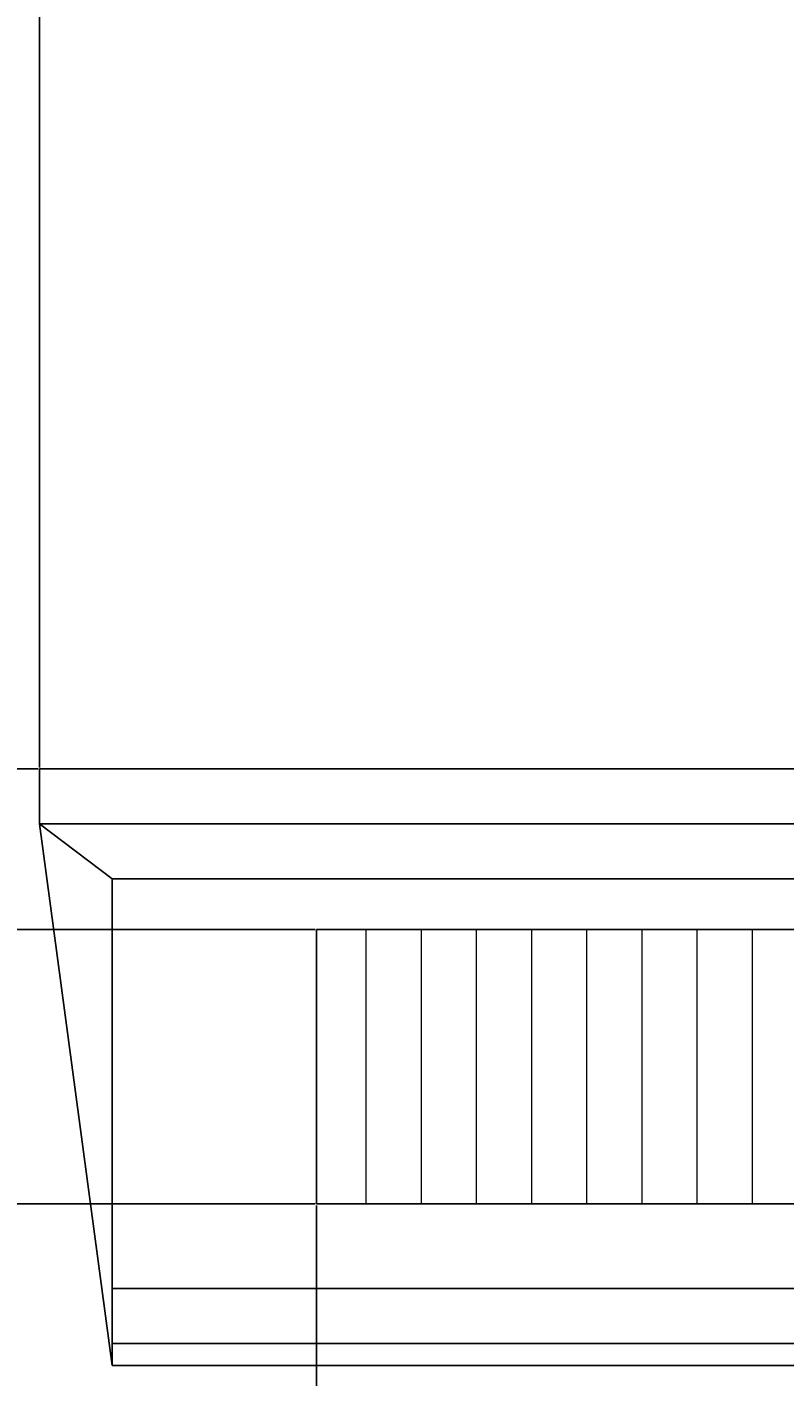
# Model space of a CAD drawing. Units: millimetres. Extents: x 2332 to 5836, y -853 to 2199.
# Tile 8 of 16: x 3641 to 3986, y 753 to 1368. Entities that reach past the tile are written whole.
import ezdxf

# ---------------------------------------------------------------- set-up
doc = ezdxf.new("R2010")
doc.units = ezdxf.units.MM
for name, color, linetype, lineweight in [('A-ANNO-DIMS', 2, 'Continuous', 18), ('A-EQPM', 7, 'Continuous', 25), ('A-EQPM-PATT', 7, 'Continuous', 13)]:
    doc.layers.add(name, color=color, linetype=linetype, lineweight=lineweight)
doc.styles.get("Standard").update_dxf_attribs({"font": 'arial.ttf'})
doc.dimstyles.new('ISO-25', dxfattribs={"dimtxt": 2.5, "dimasz": 2.5, "dimexe": 1.25, "dimexo": 0.625, "dimtad": 1, "dimtxsty": 'Standard', "dimcen": 2.5, "dimadec": 0, "dimazin": 0, "dimtfac": 1, "dimtmove": 0, "dimatfit": 3, "dimfxl": 1, "dimarcsym": 0})

# ---------------------------------------------------------------- blocks, each defined once
blk = doc.blocks.new('*D23')
at = {"layer": 'A-ANNO-DIMS', "color": 0, "lineweight": -2, "transparency": 16777216}
for p, q in [((3646.47, 1030.43), (3646.47, 2168.7)), ((3648.97, 2167.45), (4771.11, 2167.45)), ((4773.61, 1030.43), (4773.61, 2168.7))]:
    blk.add_line(p, q, dxfattribs=at)
at = {"layer": 'A-ANNO-DIMS', "color": 0, "transparency": 16777216}
for points in [[(3648.97, 2167.87), (3648.97, 2167.04), (3646.47, 2167.45)], [(4771.11, 2167.87), (4771.11, 2167.04), (4773.61, 2167.45)]]:
    blk.add_solid(points, dxfattribs=at)
at = {"layer": 'Defpoints', "color": 0, "transparency": 16777216}
for p in [(4773.61, 2167.45), (3646.47, 1029.8), (4773.61, 1029.8)]:
    blk.add_point(p, dxfattribs=at)
at = {"layer": 'A-ANNO-DIMS', "color": 0, "transparency": 16777216, "insert": (4210.04, 2169.33), "char_height": 2.5, "attachment_point": 5}
blk.add_mtext('1127.1', dxfattribs=at)
blk = doc.blocks.new('*D27')
at = {"layer": 'A-ANNO-DIMS', "color": 0, "lineweight": -2, "transparency": 16777216}
for p, q in [((3772.66, 830.99), (3772.66, -853.1)), ((4647.42, 830.99), (4647.42, -853.1)), ((3775.16, -851.85), (4644.92, -851.85))]:
    blk.add_line(p, q, dxfattribs=at)
at = {"layer": 'A-ANNO-DIMS', "color": 0, "transparency": 16777216}
for points in [[(3775.16, -851.43), (3775.16, -852.26), (3772.66, -851.85)], [(4644.92, -851.43), (4644.92, -852.26), (4647.42, -851.85)]]:
    blk.add_solid(points, dxfattribs=at)
at = {"layer": 'Defpoints', "color": 0, "transparency": 16777216}
for p in [(3772.66, 831.62), (4647.42, 831.62), (4647.42, -851.85)]:
    blk.add_point(p, dxfattribs=at)
at = {"layer": 'A-ANNO-DIMS', "color": 0, "transparency": 16777216, "insert": (4210.04, -849.95), "char_height": 2.5, "attachment_point": 5}
blk.add_mtext('874.8', dxfattribs=at)
blk = doc.blocks.new('*D28')
at = {"layer": 'A-ANNO-DIMS', "color": 0, "lineweight": -2, "transparency": 16777216}
for p, q in [((3772.04, 956.62), (2334.14, 956.62)), ((2335.39, 834.12), (2335.39, 954.12)), ((3772.04, 831.62), (2334.14, 831.62))]:
    blk.add_line(p, q, dxfattribs=at)
at = {"layer": 'A-ANNO-DIMS', "color": 0, "transparency": 16777216}
for points in [[(2334.97, 954.12), (2335.81, 954.12), (2335.39, 956.62)], [(2334.97, 834.12), (2335.81, 834.12), (2335.39, 831.62)]]:
    blk.add_solid(points, dxfattribs=at)
at = {"layer": 'Defpoints', "color": 0, "transparency": 16777216}
for p in [(2335.39, 956.62), (3772.66, 956.62), (3772.66, 831.62)]:
    blk.add_point(p, dxfattribs=at)
at = {"layer": 'A-ANNO-DIMS', "color": 0, "transparency": 16777216, "insert": (2333.49, 894.12), "char_height": 2.5, "attachment_point": 5, "rotation": 90}
blk.add_mtext('125', dxfattribs=at)
blk = doc.blocks.new('*D29')
at = {"layer": 'A-ANNO-DIMS', "color": 0, "lineweight": -2, "transparency": 16777216}
for p, q in [((3634.41, 1367.8), (2334.14, 1367.8)), ((2335.39, 1032.3), (2335.39, 1365.3)), ((3645.84, 1029.8), (2334.14, 1029.8))]:
    blk.add_line(p, q, dxfattribs=at)
at = {"layer": 'A-ANNO-DIMS', "color": 0, "transparency": 16777216}
for points in [[(2334.97, 1365.3), (2335.81, 1365.3), (2335.39, 1367.8)], [(2334.97, 1032.3), (2335.81, 1032.3), (2335.39, 1029.8)]]:
    blk.add_solid(points, dxfattribs=at)
at = {"layer": 'Defpoints', "color": 0, "transparency": 16777216}
for p in [(2335.39, 1367.8), (3635.04, 1367.8), (3646.47, 1029.8)]:
    blk.add_point(p, dxfattribs=at)
at = {"layer": 'A-ANNO-DIMS', "color": 0, "transparency": 16777216, "insert": (2333.49, 1198.8), "char_height": 2.5, "attachment_point": 5, "rotation": 90}
blk.add_mtext('338', dxfattribs=at)
blk = doc.blocks.new('*D30')
at = {"layer": 'A-ANNO-DIMS', "color": 0, "lineweight": -2, "transparency": 16777216}
for p, q in [((3635.04, 1368.43), (3635.04, 2168.7)), ((3637.54, 2167.45), (4207.54, 2167.45)), ((4210.04, 1368.43), (4210.04, 2168.7))]:
    blk.add_line(p, q, dxfattribs=at)
at = {"layer": 'A-ANNO-DIMS', "color": 0, "transparency": 16777216}
for points in [[(3637.54, 2167.87), (3637.54, 2167.04), (3635.04, 2167.45)], [(4207.54, 2167.87), (4207.54, 2167.04), (4210.04, 2167.45)]]:
    blk.add_solid(points, dxfattribs=at)
at = {"layer": 'Defpoints', "color": 0, "transparency": 16777216}
for p in [(4210.04, 2167.45), (3635.04, 1367.8), (4210.04, 1367.8)]:
    blk.add_point(p, dxfattribs=at)
at = {"layer": 'A-ANNO-DIMS', "color": 0, "transparency": 16777216, "insert": (3922.54, 2169.35), "char_height": 2.5, "attachment_point": 5}
blk.add_mtext('575', dxfattribs=at)

msp = doc.modelspace()

# ---------------------------------------------------------------- hatches: boundary and pattern name
at = {"layer": 'A-EQPM-PATT'}
h = msp.add_hatch(dxfattribs=at)
h.set_pattern_fill('ANSI31', color=256, scale=7.9164, angle=45, style=0)
h.paths.add_polyline_path([(3772.661, 831.62), (4647.419, 831.62), (4647.419, 956.62), (3772.661, 956.62)])

# ---------------------------------------------------------------- linework, layer by layer
at = {"layer": 'A-EQPM'}
for p, q in [((4079.186, 1029.801), (3646.468, 1029.801)), ((3646.468, 1029.801), (3646.468, 1004.801)), ((3646.468, 1004.801), (4210.04, 1004.801)), ((3646.468, 1004.801), (3679.541, 979.768)), ((3646.468, 1004.801), (3679.541, 758.058)), ((3679.541, 979.768), (4210.04, 979.768)), ((3679.541, 979.768), (3679.541, 758.058)), ((3772.661, 956.62), (3772.661, 831.62)), ((3772.661, 956.62), (4210.04, 956.62)), ((3772.661, 831.62), (4210.04, 831.62)), ((3679.541, 793.058), (4210.04, 793.058)), ((3679.541, 768.058), (4210.04, 768.058)), ((3679.541, 758.058), (4210.04, 758.058))]:
    msp.add_line(p, q, dxfattribs=at)

# ---------------------------------------------------------------- dimensions: what is measured, and where the dimension line sits
at = {"layer": 'A-ANNO-DIMS'}
for base, p1, p2, override, picture, middle in [((4210.04, 2167.453), (3635.04, 1367.803), (4210.04, 1367.803), {"dimdec": 0, "dimlfac": 1, "dimrnd": 0, "dimzin": 0, "dimdsep": 46, "dimlunit": 2}, '*D30', (3922.54, 2169.35)), ((4773.612, 2167.453), (3646.468, 1029.801), (4773.612, 1029.801), {"dimdec": 1, "dimlfac": 1, "dimrnd": 0, "dimzin": 0, "dimdsep": 46, "dimlunit": 2}, '*D23', (4210.04, 2169.334)), ((4647.419, -851.847), (3772.661, 831.62), (4647.419, 831.62), {"dimdec": 1, "dimlfac": 1, "dimrnd": 0, "dimzin": 0, "dimdsep": 46, "dimlunit": 2}, '*D27', (4210.04, -849.945))]:
    dim = msp.add_linear_dim(base=base, p1=p1, p2=p2, dimstyle='ISO-25', override=override, dxfattribs=at)
    dim.commit()
    dim.dimension.update_dxf_attribs({"geometry": picture, "text_midpoint": middle})
for base, p1, p2, picture, middle in [((2335.39, 1367.803), (3646.468, 1029.801), (3635.04, 1367.803), '*D29', (2333.488, 1198.802)), ((2335.39, 956.62), (3772.661, 831.62), (3772.661, 956.62), '*D28', (2333.488, 894.12))]:
    dim = msp.add_linear_dim(base=base, p1=p1, p2=p2, angle=90, dimstyle='ISO-25', override={"dimdec": 0, "dimlfac": 1, "dimrnd": 0, "dimzin": 0, "dimdsep": 46, "dimlunit": 2}, dxfattribs=at)
    dim.commit()
    dim.dimension.update_dxf_attribs({"geometry": picture, "text_midpoint": middle})

doc.saveas('drawing.dxf')
